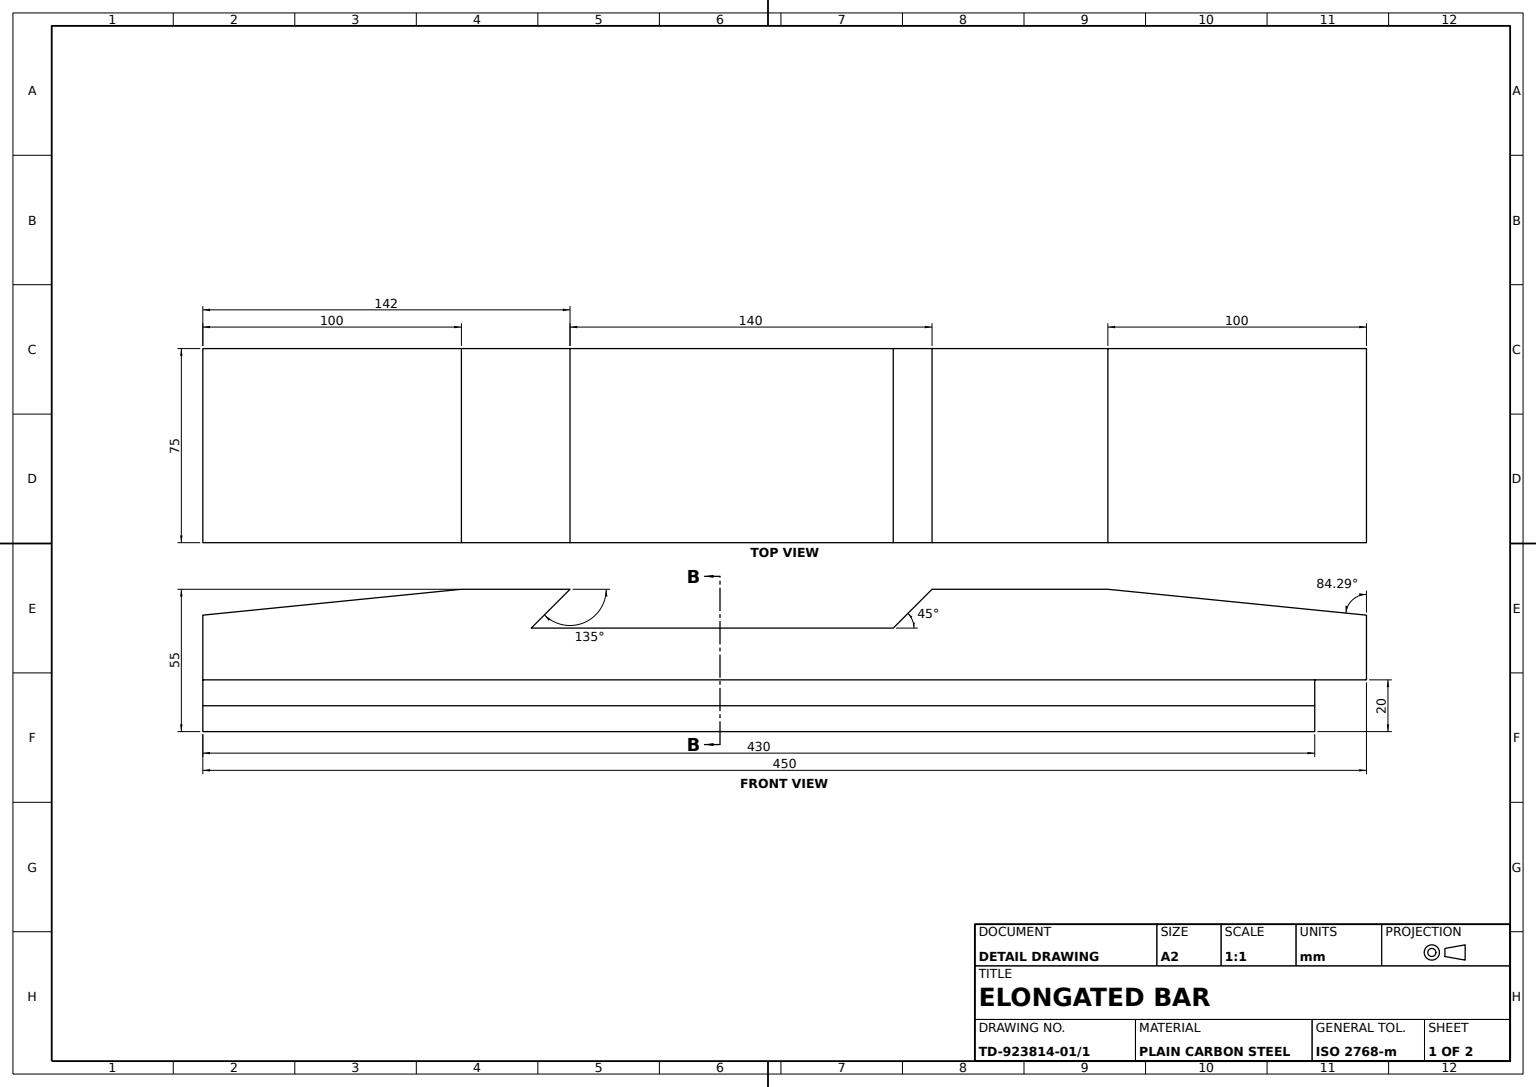
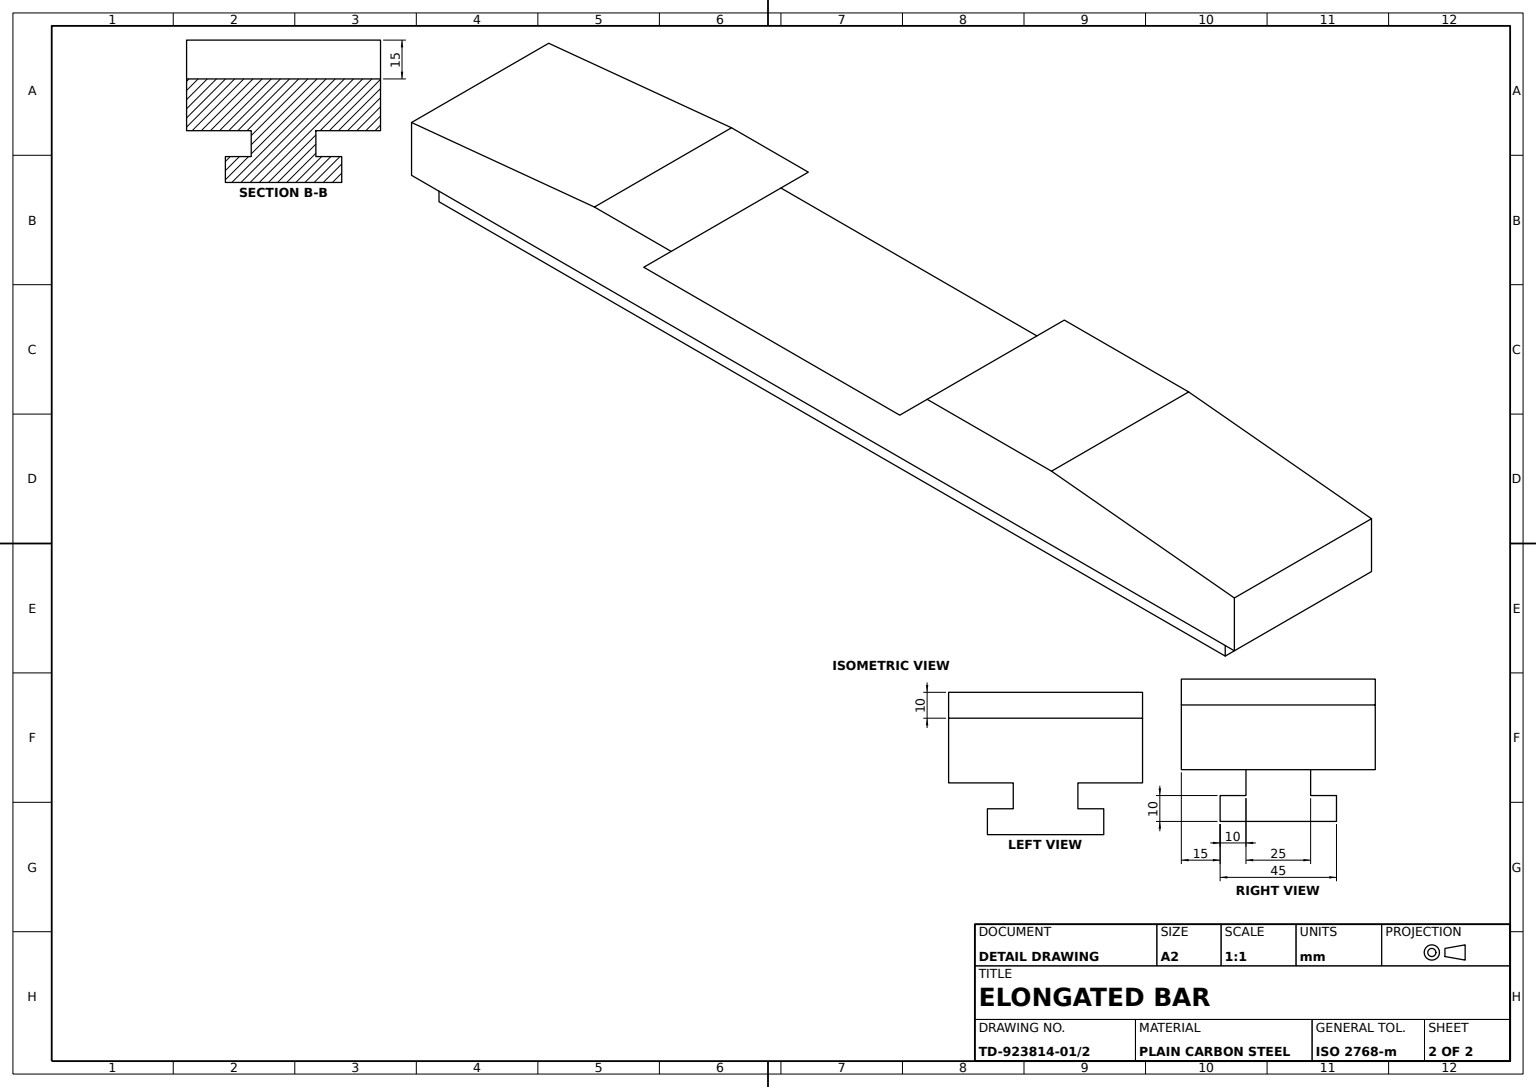
from build123d import *

# Parameters (mm, degrees)
BASE_BAR_EXTRUDE_75MM_DEPTH    = 37.5
SKETCH1_4_W                    = 430
SKETCH1_4_H                    = 10
PROFILE_REGION_BOSS_25MM_DEPTH = 12.5
SKETCH1_5_W                    = 430
SKETCH1_5_H                    = 10
PROFILE_REGION_BOSS_45MM_DEPTH = 22.5


with BuildPart() as part:
    # Bar Profile Sketch → Base Bar Extrude 75mm (new, symmetric)
    with BuildSketch(Plane.XY):
        Polygon((0, 25), (0, 0), (430, 0), (450, 0), (450, 25), (350, 35), (282, 35), (267, 20), (127, 20), (142, 35), (100, 35), align=None)
    extrude(amount=BASE_BAR_EXTRUDE_75MM_DEPTH, both=True)

    # Sketch1_4 → Profile Region Boss 25mm (add, symmetric)
    with BuildSketch(Plane.XY):
        with Locations((215, -5)):
            Rectangle(SKETCH1_4_W, SKETCH1_4_H)
    extrude(amount=PROFILE_REGION_BOSS_25MM_DEPTH, both=True)

    # Sketch1_5 → Profile Region Boss 45mm (add, symmetric)
    with BuildSketch(Plane.XY):
        with Locations((215, -15)):
            Rectangle(SKETCH1_5_W, SKETCH1_5_H)
    extrude(amount=PROFILE_REGION_BOSS_45MM_DEPTH, both=True)


solid = part.part
